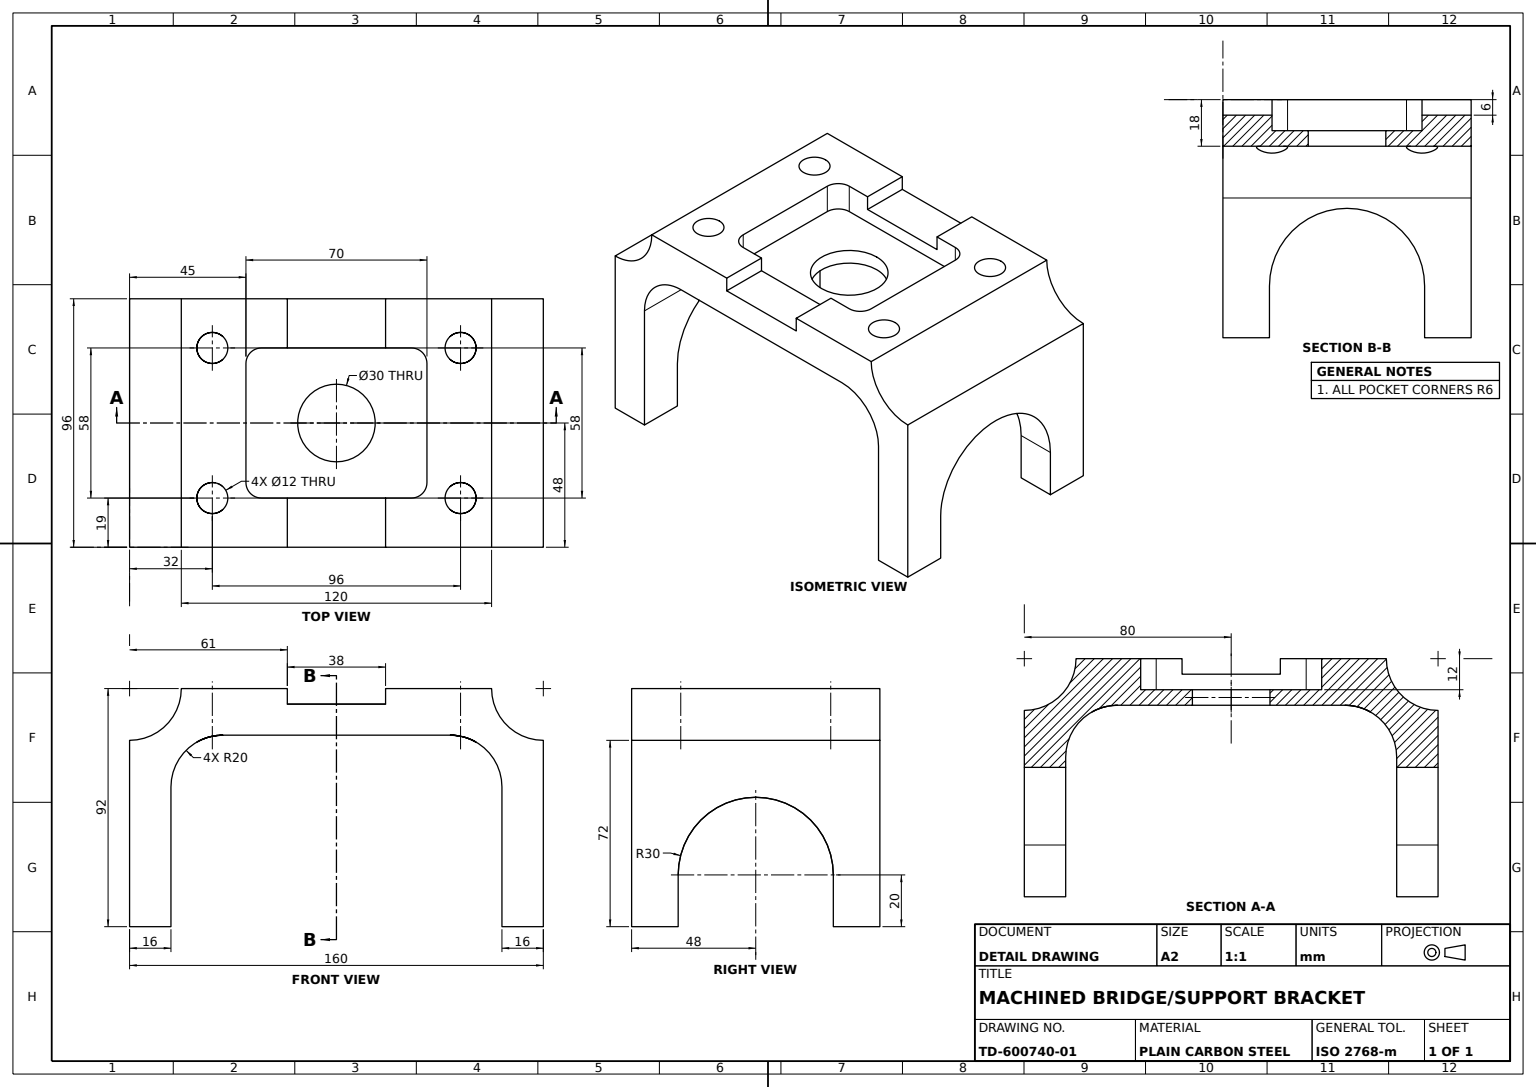
SolidWorks part; units mm, degrees
material "Plain Carbon Steel"
ref_plane "Front Plane" through (0, 0, 0) normal (0, 0, 1) x (1, 0, 0)
ref_plane "Top Plane" through (0, 0, 0) normal (0, 1, 0) x (1, 0, 0)
ref_plane "Right Plane" through (0, 0, 0) normal (1, 0, 0) x (0, 0, -1)
sketch "Bridge Profile Sketch" plane through (0, 0, 0) normal (0, 0, 1) x (1, 0, 0)
  line L0 (-80, 0) -> (-64, 0)
  line L1 (-80, 0) -> (-80, 72)
  line L2 (-60, 92) -> (60, 92)
  line L3 (80, 72) -> (80, 0)
  line L4 (-64, 0) -> (-64, 54)
  line L5 (64, 54) -> (64, 0)
  line L6 (-44, 74) -> (44, 74)
  line L7 (64, 72) -> (64, 0) construction
  line L8 (-60, 74) -> (60, 74) construction
  line L9 (-64, 0) -> (-64, 72) construction
  line L10 (64, 0) -> (80, 0)
  arc A0 (-80, 72) -> (-60, 92) centre (-80, 92) ccw
  arc A1 (60, 92) -> (80, 72) centre (80, 92) ccw
  arc A2 (64, 54) -> (44, 74) centre (44, 54) ccw
  arc A3 (-44, 74) -> (-64, 54) centre (-44, 54) ccw
  point P4 (0, 0)
  dimension "D3" = 40
  dimension "D4" = 40
  dimension "D11" = 20
  dimension "D1" = 80
  dimension "D2" = 92
  dimension "D5" = 120
  dimension "D6" = 72
  dimension "D7" = 72
  dimension "D8" = 92
  dimension "D12" = 64
  dimension "D13" = 64
  dimension "D9" = 16
  dimension "D10" = 18
extrude "Bridge Body" add sketch "Bridge Profile Sketch" along normal blind 96
sketch "Arch Relief Sketch" plane through (80, 0, 0) normal (1, 0, 0) x (0, 0, -1)
  line L0 (-96, 0) -> (0, 0) construction
  line L1 (-96, 0) -> (-96, 72) construction
  line L2 (-78, 20) -> (-78, 0)
  line L3 (-78, 0) -> (-18, 0)
  line L4 (-18, 0) -> (-18, 20)
  arc A0 (-18, 20) -> (-78, 20) centre (-48, 20) ccw
  dimension "D1" = 60
  dimension "D2" = 20
  dimension "D3" = 48
extrude "Arch Relief Cut" cut sketch "Arch Relief Sketch" against normal through all
sketch "Top Channel Sketch" plane through (0, 92, 0) normal (0, 1, 0) x (1, 0, 0)
  line L2 (-19, 0) -> (-19, -96)
  line L3 (19, 0) -> (19, -96)
  line L4 (-19, 0) -> (19, 0)
  line L5 (-19, -96) -> (19, -96)
  dimension "D1" = 96
  dimension "D2" = 38
  dimension "D5" = 19
  dimension "D6" = 38
extrude "Top Channel 38x6" cut sketch "Top Channel Sketch" against normal blind 6
sketch "Center Bore Sketch" plane through (0, 86, 0) normal (0, 1, 0) x (1, 0, 0)
  line L0 (19, 0) -> (-19, 0) construction
  line L1 (80, -96) -> (80, 0) construction
  circle A0 centre (0, -48) radius 15
  dimension "D1" = 30
  dimension "D2" = 48
  dimension "D3" = 80
extrude "Center Bore Ø30" cut sketch "Center Bore Sketch" against normal through all
sketch "Mounting Holes Sketch" plane through (0, 92, 0) normal (0, 1, 0) x (1, 0, 0)
  line L5 (-48, -77) -> (48, -19) construction
  line L6 (-48, -19) -> (48, -77) construction
  circle A0 centre (-48, -19) radius 6
  circle A1 centre (48, -19) radius 6
  circle A2 centre (48, -77) radius 6
  circle A3 centre (-48, -77) radius 6
  point P0 (0, -48)
  dimension "D1" = 12
  dimension "D2" = 12
  dimension "D3" = 12
  dimension "D4" = 12
  dimension "D5" = 58
  dimension "D6" = 29
  dimension "D7" = 48
  dimension "D8" = 29
  dimension "D9" = 48
  dimension "D10" = 48
extrude "Mounting Holes 4xØ12" cut sketch "Mounting Holes Sketch" against normal through all
sketch "Center Pocket Sketch" plane through (0, 92, 0) normal (0, 1, 0) x (1, 0, 0)
  line L1 (-29, -77) -> (29, -77)
  line L2 (-35, -71) -> (-35, -25)
  line L3 (-29, -19) -> (29, -19)
  line L4 (35, -71) -> (35, -25)
  line L5 (-35, -77) -> (35, -19) construction
  line L6 (-35, -19) -> (35, -77) construction
  arc A0 (29, -19) -> (35, -25) centre (29, -25) cw
  arc A1 (29, -77) -> (35, -71) centre (29, -71) ccw
  arc A2 (-29, -77) -> (-35, -71) centre (-29, -71) cw
  arc A3 (-35, -25) -> (-29, -19) centre (-29, -25) cw
  point P0 (0, -48)
  dimension "D3" = 6
  dimension "D1" = 58
  dimension "D2" = 70
extrude "Center Pocket 58x70" cut sketch "Center Pocket Sketch" against normal blind 12
